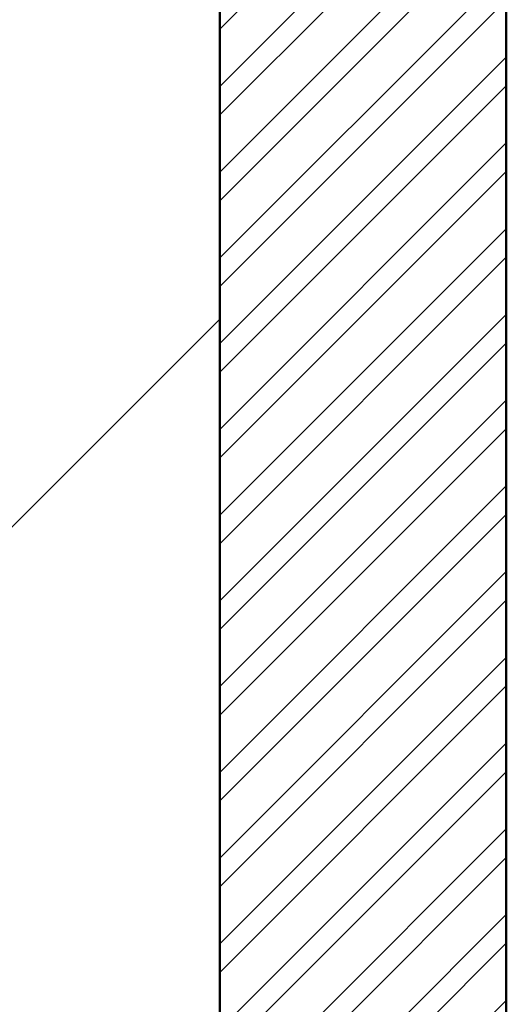
# Model space of a CAD drawing. Units: inches. Extents: x 3590 to 5167, y 65 to 1917.
# Tile 43 of 100: x 5065 to 5080, y 1357 to 1388. Entities that reach past the tile are written whole.
import ezdxf

# ---------------------------------------------------------------- set-up
doc = ezdxf.new("R2010")
doc.units = ezdxf.units.IN
for name, color, linetype, lineweight in [('A-FLOR-PATT', 8, 'Continuous', 13), ('A-WALL', 7, 'Continuous', 50), ('A-WALL-PATT', 251, 'Continuous', 13)]:
    doc.layers.add(name, color=color, linetype=linetype, lineweight=lineweight)

msp = doc.modelspace()

# ---------------------------------------------------------------- hatches: boundary and pattern name
at = {"layer": 'A-FLOR-PATT', "transparency": 33554687}
h = msp.add_hatch(dxfattribs=at)
h.set_pattern_fill('AR-HBONE', color=256, scale=0.2)
h.set_pattern_definition([(45, (-588.972, 0), (0, 28.73682), [60.96, -20.32]), (135, (-574.604, 14.368), (3e-15, 28.73682), [60.96, -20.32])])
h.paths.add_polyline_path([(5071.274, 1796.999), (4933.274, 1796.999), (4933.274, 1753.999), (4962.774, 1753.999, -0.414214), (4928.774, 1719.999), (4933.274, 1718.999), (4933.274, 1334.999), (5071.274, 1334.999)])
h.paths.add_polyline_path([(4951.78, 1521.077), (4951.715, 1521.04), (4951.563, 1520.895)], flags=16)
h.paths.add_polyline_path([(4952.267, 1521.376), (4952.198, 1521.371), (4952.198, 1521.356)], flags=0)
h.paths.add_polyline_path([(4967.051, 1529.728), (4965.231, 1528.694), (4963.411, 1527.714), (4961.756, 1526.851), (4963.589, 1527.449), (4964.036, 1527.478), (4962.975, 1527.249), (4961.76, 1526.852), (4959.792, 1525.834), (4958.005, 1524.895), (4956.24, 1523.93), (4954.504, 1522.919), (4954.129, 1522.682), (4953.361, 1521.997), (4953.366, 1521.998), (4953.605, 1522.064), (4955.106, 1522.761), (4956.921, 1523.434), (4958.678, 1523.915), (4960.358, 1524.2), (4961.945, 1524.286), (4964.171, 1524.108), (4965.958, 1523.309), (4963.863, 1522.976), (4965.187, 1522.499), (4963.366, 1522.497), (4961.545, 1522.487), (4959.764, 1522.461), (4958.304, 1522.419), (4957.974, 1522.388), (4956.307, 1522.232), (4954.718, 1522.071), (4953.251, 1521.899), (4953.525, 1521.623), (4954.331, 1521.379), (4956.243, 1521.23), (4958.039, 1520.93), (4959.684, 1520.483), (4961.16, 1519.896), (4963.107, 1518.8), (4964.393, 1517.325), (4962.973, 1517.726), (4964.558, 1516.661), (4965.407, 1515.708), (4963.507, 1516.322), (4961.68, 1517.005), (4959.935, 1517.745), (4958.282, 1518.528), (4956.732, 1519.343), (4955.295, 1520.175), (4954.672, 1520.572), (4954.513, 1520.627), (4955.658, 1519.318), (4956.703, 1517.982), (4957.644, 1516.647), (4958.485, 1515.334), (4959.55, 1513.524), (4960.438, 1511.769), (4958.841, 1513.62), (4957.452, 1515.325), (4955.819, 1517.459), (4956.665, 1515.448), (4957.111, 1513.923), (4957.447, 1511.714), (4957.076, 1509.793), (4956.538, 1511.11), (4955.992, 1512.569), (4955.444, 1514.125), (4954.898, 1515.735), (4954.357, 1517.356), (4953.824, 1518.943), (4953.305, 1520.452), (4953.065, 1521.116), (4952.971, 1521.146), (4952.949, 1521.086), (4952.73, 1520.199), (4953.37, 1518.024), (4953.757, 1516.373), (4954.051, 1514.765), (4954.264, 1513.221), (4954.471, 1511.131), (4954.497, 1510.402), (4954.409, 1511.76), (4954.264, 1513.221), (4954.051, 1514.765), (4953.757, 1516.373), (4953.37, 1518.024), (4952.877, 1519.698), (4952.716, 1520.141), (4952.533, 1519.059), (4952.374, 1517.789), (4952.219, 1516.312), (4952.046, 1514.6), (4951.833, 1512.626), (4951.557, 1510.363), (4951.203, 1512.168), (4950.852, 1514.339), (4950.985, 1516.376), (4951.66, 1518.286), (4952.593, 1520.481), (4952.357, 1521.13), (4951.855, 1520.328), (4950.839, 1518.908), (4949.777, 1517.587), (4948.916, 1516.617), (4948.111, 1515.256), (4947.089, 1513.554), (4945.889, 1511.615), (4946.326, 1513.402), (4946.562, 1514.249), (4945.528, 1513.327), (4944.581, 1512.531), (4946.018, 1514.508), (4947.204, 1516.048), (4947.893, 1517.313), (4949.307, 1518.764), (4950.414, 1519.767), (4950.451, 1519.806), (4952.267, 1521.376), (4951.645, 1521.493), (4950.404, 1521.18), (4948.044, 1520.359), (4946.119, 1519.452), (4944.572, 1518.475), (4943.35, 1517.443), (4941.997, 1515.92), (4941.661, 1515.275), (4942.813, 1516.99), (4944.572, 1518.475), (4946.119, 1519.452), (4948.044, 1520.359), (4950.404, 1521.18), (4951.645, 1521.493), (4949.647, 1521.868), (4948.6, 1521.756), (4947.126, 1521.57), (4945.42, 1521.348), (4943.45, 1521.105), (4941.183, 1520.856), (4942.86, 1521.613), (4943.873, 1522.03), (4942.952, 1521.909), (4941.41, 1521.485), (4939.543, 1520.67), (4938.968, 1520.226), (4940.733, 1521.299), (4942.952, 1521.909), (4943.702, 1522.008), (4945.894, 1522.7), (4947.565, 1522.714), (4948.921, 1522.566), (4951.131, 1522.183), (4950.971, 1522.297), (4948.129, 1523.006), (4946.035, 1523.707), (4944.232, 1524.521), (4942.707, 1525.461), (4941.444, 1526.537), (4940.43, 1527.761), (4939.649, 1529.143), (4941.421, 1528.122), (4943.147, 1527.132), (4944.841, 1526.175), (4946.514, 1525.25), (4948.179, 1524.359), (4948.365, 1524.263), (4946.475, 1526.045), (4945.181, 1527.54), (4944.19, 1529.033), (4943.496, 1530.54), (4943.278, 1531.36), (4942.498, 1531.919), (4943.114, 1531.762), (4942.959, 1533.659), (4944.14, 1531.989), (4944.612, 1531.323), (4946.202, 1530.463), (4947.486, 1529.509), (4948.79, 1528.226), (4950.368, 1526.237), (4949.485, 1528.155), (4948.851, 1530.123), (4948.491, 1532.041), (4948.381, 1533.918), (4948.501, 1535.76), (4948.827, 1537.573), (4949.418, 1535.565), (4949.957, 1533.569), (4950.464, 1531.586), (4950.961, 1529.617), (4951.391, 1527.954), (4951.724, 1530.687), (4952.201, 1532.58), (4952.889, 1534.33), (4953.77, 1535.951), (4954.827, 1537.46), (4954.521, 1535.39), (4954.273, 1533.937), (4955.58, 1535.663), (4956.748, 1536.739), (4956.159, 1534.78), (4955.589, 1532.873), (4955.043, 1531.006), (4954.525, 1529.166), (4954.038, 1527.341), (4953.638, 1525.733), (4953.611, 1525.586), (4953.398, 1524.166), (4953.382, 1524.009), (4954.07, 1525.476), (4954.912, 1527.022), (4956.136, 1528.894), (4957.847, 1530.577), (4959.376, 1531.54), (4958.256, 1530.104), (4957.143, 1528.663), (4956.066, 1527.243), (4955.056, 1525.871), (4954.141, 1524.571), (4953.352, 1523.372), (4953.311, 1523.303), (4953.273, 1522.925), (4953.261, 1522.382), (4954.103, 1523.373), (4954.63, 1524.284), (4955.961, 1526.358), (4957.23, 1528.13), (4958.421, 1529.609), (4960.037, 1531.368), (4961.374, 1532.375), (4962.101, 1532.77), (4961.07, 1531.061), (4959.987, 1529.438), (4958.869, 1527.908), (4958.15, 1527.007), (4959.803, 1528.003), (4961.589, 1528.793), (4963.391, 1529.328), (4965.211, 1529.632)], flags=16)
h.paths.add_polyline_path([(4962.944, 1523.182), (4961.107, 1523.422), (4960.392, 1523.362), (4962.35, 1523.331)], flags=0)
h.paths.add_polyline_path([(5049.541, 1584.551), (5049.476, 1584.515), (5049.325, 1584.37)], flags=16)
h.paths.add_polyline_path([(5050.028, 1584.851), (5049.959, 1584.845), (5049.959, 1584.83)], flags=0)
h.paths.add_polyline_path([(5042.333, 1581.949), (5043.88, 1582.926), (5045.806, 1583.833), (5048.165, 1584.654), (5049.406, 1584.967), (5047.408, 1585.342), (5046.361, 1585.231), (5044.888, 1585.044), (5043.181, 1584.822), (5041.211, 1584.579), (5038.944, 1584.33), (5040.622, 1585.087), (5041.634, 1585.504), (5040.713, 1585.383), (5039.171, 1584.959), (5037.304, 1584.144), (5036.729, 1583.7), (5038.494, 1584.773), (5040.713, 1585.383), (5041.463, 1585.482), (5043.655, 1586.174), (5045.326, 1586.188), (5046.682, 1586.04), (5048.893, 1585.657), (5048.732, 1585.771), (5045.891, 1586.48), (5043.796, 1587.181), (5041.994, 1587.996), (5040.468, 1588.935), (5039.205, 1590.011), (5038.191, 1591.235), (5037.41, 1592.617), (5039.182, 1591.596), (5040.909, 1590.607), (5042.602, 1589.649), (5044.275, 1588.724), (5045.94, 1587.833), (5046.126, 1587.738), (5044.237, 1589.519), (5042.942, 1591.015), (5041.952, 1592.508), (5041.257, 1594.014), (5041.039, 1594.834), (5040.26, 1595.393), (5040.875, 1595.237), (5040.721, 1597.133), (5041.901, 1595.463), (5042.373, 1594.798), (5043.963, 1593.938), (5045.247, 1592.983), (5046.552, 1591.701), (5048.129, 1589.712), (5047.247, 1591.63), (5046.613, 1593.597), (5046.252, 1595.515), (5046.142, 1597.392), (5046.262, 1599.234), (5046.588, 1601.047), (5047.179, 1599.039), (5047.718, 1597.043), (5048.225, 1595.06), (5048.722, 1593.091), (5049.152, 1591.429), (5049.485, 1594.161), (5049.962, 1596.054), (5050.65, 1597.804), (5051.532, 1599.425), (5052.589, 1600.934), (5052.283, 1598.864), (5052.034, 1597.411), (5053.341, 1599.137), (5054.509, 1600.213), (5053.92, 1598.254), (5053.35, 1596.348), (5052.805, 1594.48), (5052.286, 1592.64), (5051.799, 1590.815), (5051.4, 1589.207), (5051.373, 1589.06), (5051.159, 1587.64), (5051.143, 1587.483), (5051.831, 1588.95), (5052.673, 1590.496), (5053.898, 1592.368), (5055.608, 1594.051), (5057.137, 1595.014), (5056.017, 1593.578), (5054.904, 1592.137), (5053.828, 1590.717), (5052.817, 1589.345), (5051.902, 1588.046), (5051.113, 1586.846), (5051.072, 1586.777), (5051.034, 1586.399), (5051.022, 1585.856), (5051.864, 1586.847), (5052.391, 1587.758), (5053.723, 1589.832), (5054.991, 1591.604), (5056.182, 1593.083), (5057.798, 1594.842), (5059.135, 1595.849), (5059.863, 1596.244), (5058.831, 1594.535), (5057.749, 1592.912), (5056.63, 1591.382), (5055.912, 1590.482), (5057.564, 1591.477), (5059.35, 1592.267), (5061.152, 1592.802), (5062.972, 1593.106), (5064.812, 1593.203), (5062.992, 1592.169), (5061.172, 1591.188), (5059.518, 1590.325), (5061.35, 1590.924), (5061.797, 1590.952), (5060.737, 1590.723), (5059.521, 1590.326), (5057.553, 1589.308), (5055.766, 1588.369), (5054.002, 1587.404), (5052.265, 1586.393), (5051.891, 1586.156), (5051.122, 1585.471), (5051.127, 1585.472), (5051.366, 1585.538), (5052.867, 1586.235), (5054.682, 1586.908), (5056.439, 1587.389), (5058.12, 1587.675), (5059.706, 1587.76), (5061.933, 1587.583), (5063.719, 1586.783), (5061.624, 1586.45), (5062.949, 1585.973), (5061.127, 1585.971), (5059.307, 1585.961), (5057.525, 1585.935), (5056.065, 1585.893), (5055.735, 1585.862), (5054.068, 1585.707), (5052.479, 1585.546), (5051.012, 1585.373), (5051.286, 1585.097), (5052.092, 1584.853), (5054.004, 1584.704), (5055.8, 1584.404), (5057.446, 1583.958), (5058.921, 1583.37), (5060.868, 1582.274), (5062.154, 1580.799), (5060.734, 1581.2), (5062.32, 1580.135), (5063.168, 1579.182), (5061.269, 1579.796), (5059.441, 1580.479), (5057.696, 1581.219), (5056.043, 1582.003), (5054.493, 1582.817), (5053.057, 1583.649), (5052.433, 1584.047), (5052.274, 1584.101), (5053.42, 1582.793), (5054.464, 1581.457), (5055.405, 1580.121), (5056.247, 1578.809), (5057.311, 1576.998), (5058.199, 1575.244), (5056.602, 1577.094), (5055.213, 1578.799), (5053.58, 1580.933), (5054.427, 1578.922), (5054.872, 1577.397), (5055.208, 1575.189), (5054.838, 1573.267), (5054.299, 1574.584), (5053.754, 1576.043), (5053.206, 1577.599), (5052.659, 1579.209), (5052.118, 1580.83), (5051.585, 1582.417), (5051.066, 1583.927), (5050.826, 1584.59), (5050.733, 1584.62), (5050.711, 1584.561), (5050.491, 1583.673), (5051.131, 1581.498), (5051.518, 1579.847), (5051.813, 1578.24), (5052.026, 1576.695), (5052.233, 1574.605), (5052.258, 1573.876), (5052.17, 1575.234), (5052.026, 1576.695), (5051.813, 1578.24), (5051.518, 1579.847), (5051.131, 1581.498), (5050.638, 1583.172), (5050.477, 1583.615), (5050.294, 1582.533), (5050.136, 1581.263), (5049.981, 1579.786), (5049.807, 1578.074), (5049.594, 1576.1), (5049.318, 1573.837), (5048.965, 1575.642), (5048.613, 1577.813), (5048.747, 1579.85), (5049.421, 1581.76), (5050.354, 1583.955), (5050.118, 1584.604), (5049.616, 1583.802), (5048.6, 1582.382), (5047.538, 1581.061), (5046.677, 1580.091), (5045.872, 1578.73), (5044.85, 1577.028), (5043.651, 1575.089), (5044.087, 1576.877), (5044.324, 1577.723), (5043.289, 1576.801), (5042.342, 1576.005), (5043.779, 1577.982), (5044.966, 1579.522), (5045.655, 1580.787), (5047.068, 1582.239), (5048.175, 1583.241), (5048.213, 1583.28), (5050.028, 1584.851), (5049.406, 1584.967), (5048.165, 1584.654), (5045.806, 1583.833), (5043.88, 1582.926), (5042.333, 1581.949), (5041.111, 1580.917), (5039.758, 1579.394), (5039.423, 1578.749), (5040.575, 1580.464)], flags=16)
h.paths.add_polyline_path([(4954.799, 1533.12), (4954.262, 1532.079), (4953.831, 1530.935), (4953.505, 1529.636), (4953.283, 1528.133), (4953.167, 1526.376), (4953.156, 1524.315), (4953.277, 1521.236), (4952.802, 1521.842), (4951.557, 1521.998), (4950.976, 1521.961), (4952.661, 1521.941), (4952.802, 1521.842), (4953.152, 1523.593), (4953.167, 1526.376), (4953.283, 1528.133), (4953.609, 1530.346), (4954.456, 1532.592)], flags=0)
h.paths.add_polyline_path([(5050.563, 1585.316), (5049.318, 1585.472), (5048.737, 1585.435), (5050.422, 1585.415), (5050.563, 1585.316), (5050.914, 1587.067), (5050.928, 1589.851), (5051.045, 1591.607), (5051.371, 1593.82), (5052.217, 1596.066), (5052.56, 1596.594), (5052.024, 1595.554), (5051.592, 1594.409), (5051.266, 1593.11), (5051.045, 1591.607), (5050.928, 1589.851), (5050.918, 1587.789), (5051.038, 1584.71)], flags=0)
h.paths.add_polyline_path([(5058.153, 1586.836), (5060.111, 1586.805), (5060.705, 1586.656), (5058.868, 1586.896)], flags=0)
h.paths.add_polyline_path([(5049.541, 1430.936), (5049.476, 1430.9), (5049.325, 1430.755)], flags=16)
h.paths.add_polyline_path([(5050.028, 1431.236), (5049.959, 1431.231), (5049.959, 1431.215)], flags=0)
h.paths.add_polyline_path([(5046.588, 1447.432), (5047.179, 1445.425), (5047.718, 1443.429), (5048.225, 1441.446), (5048.722, 1439.476), (5049.152, 1437.814), (5049.485, 1440.546), (5049.962, 1442.439), (5050.65, 1444.189), (5051.532, 1445.811), (5052.589, 1447.319), (5052.283, 1445.249), (5052.034, 1443.796), (5053.341, 1445.522), (5054.509, 1446.598), (5053.92, 1444.64), (5053.35, 1442.733), (5052.805, 1440.865), (5052.286, 1439.025), (5051.799, 1437.201), (5051.4, 1435.592), (5051.373, 1435.445), (5051.159, 1434.025), (5051.143, 1433.868), (5051.831, 1435.335), (5052.673, 1436.881), (5053.898, 1438.753), (5055.608, 1440.436), (5057.137, 1441.4), (5056.017, 1439.963), (5054.904, 1438.522), (5053.828, 1437.102), (5052.817, 1435.73), (5051.902, 1434.431), (5051.113, 1433.231), (5051.072, 1433.162), (5051.034, 1432.784), (5051.022, 1432.242), (5051.864, 1433.232), (5052.391, 1434.143), (5053.723, 1436.217), (5054.991, 1437.989), (5056.182, 1439.468), (5057.798, 1441.227), (5059.135, 1442.235), (5059.863, 1442.629), (5058.831, 1440.921), (5057.749, 1439.298), (5056.63, 1437.767), (5055.912, 1436.867), (5057.564, 1437.863), (5059.35, 1438.652), (5061.152, 1439.187), (5062.972, 1439.491), (5064.812, 1439.588), (5062.992, 1438.554), (5061.172, 1437.573), (5059.518, 1436.71), (5061.35, 1437.309), (5061.797, 1437.337), (5060.737, 1437.108), (5059.521, 1436.711), (5057.553, 1435.693), (5055.766, 1434.754), (5054.002, 1433.789), (5052.265, 1432.778), (5051.891, 1432.541), (5051.122, 1431.856), (5051.127, 1431.857), (5051.366, 1431.923), (5052.867, 1432.62), (5054.682, 1433.293), (5056.439, 1433.775), (5058.12, 1434.06), (5059.706, 1434.145), (5061.933, 1433.968), (5063.719, 1433.168), (5061.624, 1432.835), (5062.949, 1432.358), (5061.127, 1432.357), (5059.307, 1432.346), (5057.525, 1432.32), (5056.065, 1432.278), (5055.735, 1432.248), (5054.068, 1432.092), (5052.479, 1431.931), (5051.012, 1431.759), (5051.286, 1431.482), (5052.092, 1431.238), (5054.004, 1431.089), (5055.8, 1430.789), (5057.446, 1430.343), (5058.921, 1429.755), (5060.868, 1428.66), (5062.154, 1427.185), (5060.734, 1427.585), (5062.32, 1426.52), (5063.168, 1425.567), (5061.269, 1426.181), (5059.441, 1426.865), (5057.696, 1427.604), (5056.043, 1428.388), (5054.493, 1429.202), (5053.057, 1430.034), (5052.433, 1430.432), (5052.274, 1430.487), (5053.42, 1429.178), (5054.464, 1427.842), (5055.405, 1426.506), (5056.247, 1425.194), (5057.311, 1423.383), (5058.199, 1421.629), (5056.602, 1423.479), (5055.213, 1425.184), (5053.58, 1427.318), (5054.427, 1425.307), (5054.872, 1423.782), (5055.208, 1421.574), (5054.838, 1419.652), (5054.299, 1420.97), (5053.754, 1422.428), (5053.206, 1423.984), (5052.659, 1425.595), (5052.118, 1427.215), (5051.585, 1428.802), (5051.066, 1430.312), (5050.826, 1430.975), (5050.733, 1431.005), (5050.711, 1430.946), (5050.491, 1430.058), (5051.131, 1427.883), (5051.518, 1426.232), (5051.813, 1424.625), (5052.026, 1423.081), (5052.233, 1420.991), (5052.258, 1420.261), (5052.17, 1421.619), (5052.026, 1423.081), (5051.813, 1424.625), (5051.518, 1426.232), (5051.131, 1427.883), (5050.638, 1429.558), (5050.477, 1430.001), (5050.294, 1428.918), (5050.136, 1427.648), (5049.981, 1426.171), (5049.807, 1424.459), (5049.594, 1422.485), (5049.318, 1420.222), (5048.965, 1422.028), (5048.613, 1424.199), (5048.747, 1426.235), (5049.421, 1428.146), (5050.354, 1430.34), (5050.118, 1430.989), (5049.616, 1430.187), (5048.6, 1428.768), (5047.538, 1427.446), (5046.677, 1426.477), (5045.872, 1425.116), (5044.85, 1423.413), (5043.651, 1421.474), (5044.087, 1423.262), (5044.324, 1424.109), (5043.289, 1423.186), (5042.342, 1422.391), (5043.779, 1424.368), (5044.966, 1425.907), (5045.655, 1427.173), (5047.068, 1428.624), (5048.175, 1429.627), (5048.213, 1429.666), (5050.028, 1431.236), (5049.406, 1431.353), (5048.165, 1431.039), (5045.806, 1430.218), (5043.88, 1429.311), (5042.333, 1428.334), (5041.111, 1427.302), (5039.758, 1425.779), (5039.423, 1425.134), (5040.575, 1426.849), (5042.333, 1428.334), (5043.88, 1429.311), (5045.806, 1430.218), (5048.165, 1431.039), (5049.406, 1431.353), (5047.408, 1431.727), (5046.361, 1431.616), (5044.888, 1431.429), (5043.181, 1431.207), (5041.211, 1430.964), (5038.944, 1430.715), (5040.622, 1431.472), (5041.634, 1431.89), (5040.713, 1431.769), (5039.171, 1431.345), (5037.304, 1430.53), (5036.729, 1430.085), (5038.494, 1431.158), (5040.713, 1431.769), (5041.463, 1431.867), (5043.655, 1432.559), (5045.326, 1432.573), (5046.682, 1432.425), (5048.893, 1432.042), (5048.732, 1432.156), (5045.891, 1432.865), (5043.796, 1433.566), (5041.994, 1434.381), (5040.468, 1435.321), (5039.205, 1436.396), (5038.191, 1437.62), (5037.41, 1439.002), (5039.182, 1437.982), (5040.909, 1436.992), (5042.602, 1436.034), (5044.275, 1435.109), (5045.94, 1434.218), (5046.126, 1434.123), (5044.237, 1435.904), (5042.942, 1437.4), (5041.952, 1438.893), (5041.257, 1440.399), (5041.039, 1441.219), (5040.26, 1441.778), (5040.875, 1441.622), (5040.721, 1443.518), (5041.901, 1441.848), (5042.373, 1441.183), (5043.963, 1440.323), (5045.247, 1439.369), (5046.552, 1438.086), (5048.129, 1436.097), (5047.247, 1438.015), (5046.613, 1439.982), (5046.252, 1441.901), (5046.142, 1443.778), (5046.262, 1445.619)], flags=16)
h.paths.add_polyline_path([(5052.382, 1444.255), (5051.623, 1442.78), (5052.024, 1441.939), (5052.56, 1442.98)], flags=0)
h.paths.add_polyline_path([(5050.563, 1431.701), (5049.318, 1431.857), (5048.737, 1431.821), (5050.422, 1431.8)], flags=0)
h.paths.add_polyline_path([(5058.153, 1433.221), (5060.111, 1433.19), (5060.705, 1433.041), (5058.868, 1433.281)], flags=0)
h.paths.add_polyline_path([(5049.541, 1352.285), (5049.476, 1352.249), (5049.325, 1352.104)], flags=16)
h.paths.add_polyline_path([(5050.028, 1352.585), (5049.959, 1352.58), (5049.959, 1352.564)], flags=0)
h.paths.add_polyline_path([(5046.588, 1368.781), (5047.179, 1366.774), (5047.718, 1364.778), (5048.225, 1362.795), (5048.722, 1360.825), (5049.152, 1359.163), (5049.485, 1361.896), (5049.962, 1363.789), (5050.65, 1365.538), (5051.532, 1367.16), (5052.589, 1368.669), (5052.283, 1366.598), (5052.034, 1365.145), (5053.341, 1366.871), (5054.509, 1367.947), (5053.92, 1365.989), (5053.35, 1364.082), (5052.805, 1362.214), (5052.286, 1360.374), (5051.799, 1358.55), (5051.4, 1356.942), (5051.373, 1356.794), (5051.159, 1355.374), (5051.143, 1355.218), (5051.831, 1356.684), (5052.673, 1358.23), (5053.898, 1360.102), (5055.608, 1361.786), (5057.137, 1362.749), (5056.017, 1361.313), (5054.904, 1359.872), (5053.828, 1358.452), (5052.817, 1357.079), (5051.902, 1355.78), (5051.113, 1354.581), (5051.072, 1354.512), (5051.034, 1354.133), (5051.022, 1353.591), (5051.864, 1354.581), (5052.391, 1355.492), (5053.723, 1357.566), (5054.991, 1359.338), (5056.182, 1360.817), (5057.798, 1362.577), (5059.135, 1363.584), (5059.863, 1363.979), (5058.831, 1362.27), (5057.749, 1360.647), (5056.63, 1359.117), (5055.912, 1358.216), (5057.564, 1359.212), (5059.35, 1360.001), (5061.152, 1360.536), (5062.972, 1360.841), (5064.812, 1360.937), (5062.992, 1359.903), (5061.172, 1358.923), (5059.518, 1358.059), (5061.35, 1358.658), (5061.797, 1358.687), (5060.737, 1358.458), (5059.521, 1358.061), (5057.553, 1357.043), (5055.766, 1356.103), (5054.002, 1355.138), (5052.265, 1354.127), (5051.891, 1353.89), (5051.122, 1353.206), (5051.127, 1353.206), (5051.366, 1353.272), (5052.867, 1353.969), (5054.682, 1354.643), (5056.439, 1355.124), (5058.12, 1355.409), (5059.706, 1355.495), (5061.933, 1355.317), (5063.719, 1354.518), (5061.624, 1354.184), (5062.949, 1353.708), (5061.127, 1353.706), (5059.307, 1353.695), (5057.525, 1353.669), (5056.065, 1353.627), (5055.735, 1353.597), (5054.068, 1353.441), (5052.479, 1353.28), (5051.012, 1353.108), (5051.286, 1352.831), (5052.092, 1352.587), (5054.004, 1352.439), (5055.8, 1352.138), (5057.446, 1351.692), (5058.921, 1351.104), (5060.868, 1350.009), (5062.154, 1348.534), (5060.734, 1348.935), (5062.32, 1347.869), (5063.168, 1346.916), (5061.269, 1347.53), (5059.441, 1348.214), (5057.696, 1348.954), (5056.043, 1349.737), (5054.493, 1350.551), (5053.057, 1351.383), (5052.433, 1351.781), (5052.274, 1351.836), (5053.42, 1350.527), (5054.464, 1349.191), (5055.405, 1347.855), (5056.247, 1346.543), (5057.311, 1344.733), (5058.199, 1342.978), (5056.602, 1344.828), (5055.213, 1346.534), (5053.58, 1348.667), (5054.427, 1346.656), (5054.872, 1345.132), (5055.208, 1342.923), (5054.838, 1341.002), (5054.299, 1342.319), (5053.754, 1343.778), (5053.206, 1345.334), (5052.659, 1346.944), (5052.118, 1348.564), (5051.585, 1350.151), (5051.066, 1351.661), (5050.826, 1352.324), (5050.733, 1352.355), (5050.711, 1352.295), (5050.491, 1351.408), (5051.131, 1349.232), (5051.518, 1347.581), (5051.813, 1345.974), (5052.026, 1344.43), (5052.233, 1342.34), (5052.258, 1341.61), (5052.17, 1342.969), (5052.026, 1344.43), (5051.813, 1345.974), (5051.518, 1347.581), (5051.131, 1349.232), (5050.638, 1350.907), (5050.477, 1351.35), (5050.294, 1350.267), (5050.136, 1348.997), (5049.981, 1347.52), (5049.807, 1345.809), (5049.594, 1343.835), (5049.318, 1341.571), (5048.965, 1343.377), (5048.613, 1345.548), (5048.747, 1347.585), (5049.421, 1349.495), (5050.354, 1351.689), (5050.118, 1352.339), (5049.616, 1351.536), (5048.6, 1350.117), (5047.538, 1348.795), (5046.677, 1347.826), (5045.872, 1346.465), (5044.85, 1344.763), (5043.651, 1342.824), (5044.087, 1344.611), (5044.324, 1345.458), (5043.289, 1344.535), (5042.342, 1343.74), (5043.779, 1345.717), (5044.966, 1347.256), (5045.655, 1348.522), (5047.068, 1349.973), (5048.175, 1350.976), (5048.213, 1351.015), (5050.028, 1352.585), (5049.406, 1352.702), (5048.165, 1352.388), (5045.806, 1351.567), (5043.88, 1350.661), (5042.333, 1349.683), (5041.111, 1348.651), (5039.758, 1347.128), (5039.423, 1346.483), (5040.575, 1348.198), (5042.333, 1349.683), (5043.88, 1350.661), (5045.806, 1351.567), (5048.165, 1352.388), (5049.406, 1352.702), (5047.408, 1353.076), (5046.361, 1352.965), (5044.888, 1352.779), (5043.181, 1352.556), (5041.211, 1352.313), (5038.944, 1352.065), (5040.622, 1352.821), (5041.634, 1353.239), (5040.713, 1353.118), (5039.171, 1352.694), (5037.304, 1351.879), (5036.729, 1351.434), (5038.494, 1352.508), (5040.713, 1353.118), (5041.463, 1353.216), (5043.655, 1353.909), (5045.326, 1353.923), (5046.682, 1353.774), (5048.893, 1353.391), (5048.732, 1353.506), (5045.891, 1354.214), (5043.796, 1354.915), (5041.994, 1355.73), (5040.468, 1356.67), (5039.205, 1357.746), (5038.191, 1358.969), (5037.41, 1360.352), (5039.182, 1359.331), (5040.909, 1358.341), (5042.602, 1357.383), (5044.275, 1356.458), (5045.94, 1355.567), (5046.126, 1355.472), (5044.237, 1357.253), (5042.942, 1358.749), (5041.952, 1360.242), (5041.257, 1361.748), (5041.039, 1362.568), (5040.26, 1363.128), (5040.875, 1362.971), (5040.721, 1364.867), (5041.901, 1363.197), (5042.373, 1362.532), (5043.963, 1361.672), (5045.247, 1360.718), (5046.552, 1359.435), (5048.129, 1357.446), (5047.247, 1359.364), (5046.613, 1361.331), (5046.252, 1363.25), (5046.142, 1365.127), (5046.262, 1366.969)], flags=16)
h.paths.add_polyline_path([(5052.382, 1365.604), (5051.623, 1364.129), (5052.024, 1363.288), (5052.56, 1364.329)], flags=0)
h.paths.add_polyline_path([(4951.78, 1698.041), (4951.715, 1698.005), (4951.563, 1697.859)], flags=16)
h.paths.add_polyline_path([(4952.267, 1698.341), (4952.198, 1698.335), (4952.198, 1698.32)], flags=0)
h.paths.add_polyline_path([(4957.076, 1686.757), (4956.538, 1688.074), (4955.992, 1689.533), (4955.444, 1691.089), (4954.898, 1692.699), (4954.357, 1694.32), (4953.824, 1695.907), (4953.305, 1697.417), (4953.065, 1698.08), (4952.971, 1698.11), (4952.949, 1698.051), (4952.73, 1697.163), (4953.37, 1694.988), (4953.757, 1693.337), (4954.051, 1691.729), (4954.264, 1690.185), (4954.471, 1688.095), (4954.497, 1687.366), (4954.409, 1688.724), (4954.264, 1690.185), (4954.051, 1691.729), (4953.757, 1693.337), (4953.37, 1694.988), (4952.877, 1696.662), (4952.716, 1697.105), (4952.533, 1696.023), (4952.374, 1694.753), (4952.219, 1693.276), (4952.046, 1691.564), (4951.833, 1689.59), (4951.557, 1687.327), (4951.203, 1689.132), (4950.852, 1691.303), (4950.985, 1693.34), (4951.66, 1695.25), (4952.593, 1697.445), (4952.357, 1698.094), (4951.855, 1697.292), (4950.839, 1695.872), (4949.777, 1694.551), (4948.916, 1693.581), (4948.111, 1692.22), (4947.089, 1690.518), (4945.889, 1688.579), (4946.326, 1690.366), (4946.562, 1691.213), (4945.528, 1690.291), (4944.581, 1689.495), (4946.018, 1691.472), (4947.204, 1693.012), (4947.893, 1694.277), (4949.307, 1695.729), (4950.414, 1696.731), (4950.451, 1696.77), (4952.267, 1698.341), (4951.645, 1698.457), (4950.404, 1698.144), (4948.044, 1697.323), (4946.119, 1696.416), (4944.572, 1695.439), (4943.35, 1694.407), (4941.997, 1692.884), (4941.661, 1692.239), (4942.813, 1693.954), (4944.572, 1695.439), (4946.119, 1696.416), (4948.044, 1697.323), (4950.404, 1698.144), (4951.645, 1698.457), (4949.647, 1698.832), (4948.6, 1698.72), (4947.126, 1698.534), (4945.42, 1698.312), (4943.45, 1698.069), (4941.183, 1697.82), (4942.86, 1698.577), (4943.873, 1698.994), (4942.952, 1698.873), (4941.41, 1698.449), (4939.543, 1697.634), (4938.968, 1697.19), (4940.733, 1698.263), (4942.952, 1698.873), (4943.702, 1698.972), (4945.894, 1699.664), (4947.565, 1699.678), (4948.921, 1699.53), (4951.131, 1699.147), (4950.971, 1699.261), (4948.129, 1699.97), (4946.035, 1700.671), (4944.232, 1701.486), (4942.707, 1702.425), (4941.444, 1703.501), (4940.43, 1704.725), (4939.649, 1706.107), (4941.421, 1705.086), (4943.147, 1704.097), (4944.841, 1703.139), (4946.514, 1702.214), (4948.179, 1701.323), (4948.365, 1701.227), (4946.475, 1703.009), (4945.181, 1704.505), (4944.19, 1705.997), (4943.496, 1707.504), (4943.278, 1708.324), (4942.498, 1708.883), (4943.114, 1708.727), (4942.959, 1710.623), (4944.14, 1708.953), (4944.612, 1708.287), (4946.202, 1707.428), (4947.486, 1706.473), (4948.79, 1705.191), (4950.368, 1703.202), (4949.485, 1705.12), (4948.851, 1707.087), (4948.491, 1709.005), (4948.381, 1710.882), (4948.501, 1712.724), (4948.827, 1714.537), (4949.418, 1712.529), (4949.957, 1710.533), (4950.464, 1708.55), (4950.961, 1706.581), (4951.391, 1704.919), (4951.724, 1707.651), (4952.201, 1709.544), (4952.889, 1711.294), (4953.77, 1712.915), (4954.827, 1714.424), (4954.521, 1712.354), (4954.273, 1710.901), (4955.58, 1712.627), (4956.748, 1713.703), (4956.159, 1711.744), (4955.589, 1709.837), (4955.043, 1707.97), (4954.525, 1706.13), (4954.038, 1704.305), (4953.638, 1702.697), (4953.611, 1702.55), (4953.398, 1701.13), (4953.382, 1700.973), (4954.07, 1702.44), (4954.912, 1703.986), (4956.136, 1705.858), (4957.847, 1707.541), (4959.376, 1708.504), (4958.256, 1707.068), (4957.143, 1705.627), (4956.066, 1704.207), (4955.056, 1702.835), (4954.141, 1701.536), (4953.352, 1700.336), (4953.311, 1700.267), (4953.273, 1699.889), (4953.261, 1699.346), (4954.103, 1700.337), (4954.63, 1701.248), (4955.961, 1703.322), (4957.23, 1705.094), (4958.421, 1706.573), (4960.037, 1708.332), (4961.374, 1709.339), (4962.101, 1709.734), (4961.07, 1708.025), (4959.987, 1706.402), (4958.869, 1704.872), (4958.15, 1703.972), (4959.803, 1704.967), (4961.589, 1705.757), (4963.391, 1706.292), (4965.211, 1706.596), (4967.051, 1706.692), (4965.231, 1705.659), (4963.411, 1704.678), (4961.756, 1703.815), (4963.589, 1704.413), (4964.036, 1704.442), (4962.975, 1704.213), (4961.76, 1703.816), (4959.792, 1702.798), (4958.005, 1701.859), (4956.24, 1700.894), (4954.504, 1699.883), (4954.129, 1699.646), (4953.361, 1698.961), (4953.366, 1698.962), (4953.605, 1699.028), (4955.106, 1699.725), (4956.921, 1700.398), (4958.678, 1700.879), (4960.358, 1701.164), (4961.945, 1701.25), (4964.171, 1701.073), (4965.958, 1700.273), (4963.863, 1699.94), (4965.187, 1699.463), (4963.366, 1699.461), (4961.545, 1699.451), (4959.764, 1699.425), (4958.304, 1699.383), (4957.974, 1699.352), (4956.307, 1699.197), (4954.718, 1699.036), (4953.251, 1698.863), (4953.525, 1698.587), (4954.331, 1698.343), (4956.243, 1698.194), (4958.039, 1697.894), (4959.684, 1697.447), (4961.16, 1696.86), (4963.107, 1695.764), (4964.393, 1694.289), (4962.973, 1694.69), (4964.558, 1693.625), (4965.407, 1692.672), (4963.507, 1693.286), (4961.68, 1693.969), (4959.935, 1694.709), (4958.282, 1695.492), (4956.732, 1696.307), (4955.295, 1697.139), (4954.672, 1697.536), (4954.513, 1697.591), (4955.658, 1696.282), (4956.703, 1694.946), (4957.644, 1693.611), (4958.485, 1692.298), (4959.55, 1690.488), (4960.438, 1688.733), (4958.841, 1690.584), (4957.452, 1692.289), (4955.819, 1694.423), (4956.665, 1692.412), (4957.111, 1690.887), (4957.447, 1688.678)], flags=16)
h.paths.add_polyline_path([(5050.563, 1353.05), (5049.318, 1353.207), (5048.737, 1353.17), (5050.422, 1353.15)], flags=0)
h.paths.add_polyline_path([(4951.78, 1351.486), (4951.715, 1351.45), (4951.563, 1351.305)], flags=16)
h.paths.add_polyline_path([(4952.267, 1351.786), (4952.198, 1351.78), (4952.198, 1351.765)], flags=0)
h.paths.add_polyline_path([(4954.827, 1367.869), (4954.521, 1365.799), (4954.273, 1364.346), (4955.58, 1366.072), (4956.748, 1367.148), (4956.159, 1365.19), (4955.589, 1363.283), (4955.043, 1361.415), (4954.525, 1359.575), (4954.038, 1357.751), (4953.638, 1356.142), (4953.611, 1355.995), (4953.398, 1354.575), (4953.382, 1354.418), (4954.07, 1355.885), (4954.912, 1357.431), (4956.136, 1359.303), (4957.847, 1360.986), (4959.376, 1361.95), (4958.256, 1360.513), (4957.143, 1359.072), (4956.066, 1357.652), (4955.056, 1356.28), (4954.141, 1354.981), (4953.352, 1353.781), (4953.311, 1353.712), (4953.273, 1353.334), (4953.261, 1352.792), (4954.103, 1353.782), (4954.63, 1354.693), (4955.961, 1356.767), (4957.23, 1358.539), (4958.421, 1360.018), (4960.037, 1361.777), (4961.374, 1362.785), (4962.101, 1363.179), (4961.07, 1361.471), (4959.987, 1359.848), (4958.869, 1358.317), (4958.15, 1357.417), (4959.803, 1358.413), (4961.589, 1359.202), (4963.391, 1359.737), (4965.211, 1360.041), (4967.051, 1360.138), (4965.231, 1359.104), (4963.411, 1358.123), (4961.756, 1357.26), (4963.589, 1357.859), (4964.036, 1357.887), (4962.975, 1357.658), (4961.76, 1357.261), (4959.792, 1356.243), (4958.005, 1355.304), (4956.24, 1354.339), (4954.504, 1353.328), (4954.129, 1353.091), (4953.361, 1352.406), (4953.366, 1352.407), (4953.605, 1352.473), (4955.106, 1353.17), (4956.921, 1353.843), (4958.678, 1354.325), (4960.358, 1354.61), (4961.945, 1354.695), (4964.171, 1354.518), (4965.958, 1353.718), (4963.863, 1353.385), (4965.187, 1352.908), (4963.366, 1352.907), (4961.545, 1352.896), (4959.764, 1352.87), (4958.304, 1352.828), (4957.974, 1352.798), (4956.307, 1352.642), (4954.718, 1352.481), (4953.251, 1352.309), (4953.525, 1352.032), (4954.331, 1351.788), (4956.243, 1351.639), (4958.039, 1351.339), (4959.684, 1350.893), (4961.16, 1350.305), (4963.107, 1349.21), (4964.393, 1347.735), (4962.973, 1348.135), (4964.558, 1347.07), (4965.407, 1346.117), (4963.507, 1346.731), (4961.68, 1347.414), (4959.935, 1348.154), (4958.282, 1348.938), (4956.732, 1349.752), (4955.295, 1350.584), (4954.672, 1350.982), (4954.513, 1351.036), (4955.658, 1349.728), (4956.703, 1348.392), (4957.644, 1347.056), (4958.485, 1345.744), (4959.55, 1343.933), (4960.438, 1342.179), (4958.841, 1344.029), (4957.452, 1345.734), (4955.819, 1347.868), (4956.665, 1345.857), (4957.111, 1344.332), (4957.447, 1342.124), (4957.076, 1340.202), (4956.538, 1341.52), (4955.992, 1342.978), (4955.444, 1344.534), (4954.898, 1346.145), (4954.357, 1347.765), (4953.824, 1349.352), (4953.305, 1350.862), (4953.065, 1351.525), (4952.971, 1351.555), (4952.949, 1351.496), (4952.73, 1350.608), (4953.37, 1348.433), (4953.757, 1346.782), (4954.051, 1345.175), (4954.264, 1343.631), (4954.471, 1341.541), (4954.497, 1340.811), (4954.409, 1342.169), (4954.264, 1343.631), (4954.051, 1345.175), (4953.757, 1346.782), (4953.37, 1348.433), (4952.877, 1350.108), (4952.716, 1350.551), (4952.533, 1349.468), (4952.374, 1348.198), (4952.219, 1346.721), (4952.046, 1345.009), (4951.833, 1343.035), (4951.557, 1340.772), (4951.203, 1342.578), (4950.852, 1344.749), (4950.985, 1346.785), (4951.66, 1348.696), (4952.593, 1350.89), (4952.357, 1351.539), (4951.855, 1350.737), (4950.839, 1349.318), (4949.777, 1347.996), (4948.916, 1347.027), (4948.111, 1345.665), (4947.089, 1343.963), (4945.889, 1342.024), (4946.326, 1343.812), (4946.562, 1344.659), (4945.528, 1343.736), (4944.581, 1342.941), (4946.018, 1344.918), (4947.204, 1346.457), (4947.893, 1347.723), (4949.307, 1349.174), (4950.414, 1350.177), (4950.451, 1350.216), (4952.267, 1351.786), (4951.645, 1351.903), (4950.404, 1351.589), (4948.044, 1350.768), (4946.119, 1349.861), (4944.572, 1348.884), (4943.35, 1347.852), (4941.997, 1346.329), (4941.661, 1345.684), (4942.813, 1347.399), (4944.572, 1348.884), (4946.119, 1349.861), (4948.044, 1350.768), (4950.404, 1351.589), (4951.645, 1351.903), (4949.647, 1352.277), (4948.6, 1352.166), (4947.126, 1351.979), (4945.42, 1351.757), (4943.45, 1351.514), (4941.183, 1351.265), (4942.86, 1352.022), (4943.873, 1352.44), (4942.952, 1352.319), (4941.41, 1351.895), (4939.543, 1351.08), (4938.968, 1350.635), (4940.733, 1351.708), (4942.952, 1352.319), (4943.702, 1352.417), (4945.894, 1353.109), (4947.565, 1353.123), (4948.921, 1352.975), (4951.131, 1352.592), (4950.971, 1352.706), (4948.129, 1353.415), (4946.035, 1354.116), (4944.232, 1354.931), (4942.707, 1355.871), (4941.444, 1356.946), (4940.43, 1358.17), (4939.649, 1359.552), (4941.421, 1358.532), (4943.147, 1357.542), (4944.841, 1356.584), (4946.514, 1355.659), (4948.179, 1354.768), (4948.365, 1354.673), (4946.475, 1356.454), (4945.181, 1357.95), (4944.19, 1359.443), (4943.496, 1360.949), (4943.278, 1361.769), (4942.498, 1362.328), (4943.114, 1362.172), (4942.959, 1364.068), (4944.14, 1362.398), (4944.612, 1361.733), (4946.202, 1360.873), (4947.486, 1359.919), (4948.79, 1358.636), (4950.368, 1356.647), (4949.485, 1358.565), (4948.851, 1360.532), (4948.491, 1362.451), (4948.381, 1364.328), (4948.501, 1366.169), (4948.827, 1367.982), (4949.418, 1365.975), (4949.957, 1363.979), (4950.464, 1361.995), (4950.961, 1360.026), (4951.391, 1358.364), (4951.724, 1361.096), (4952.201, 1362.989), (4952.889, 1364.739), (4953.77, 1366.361)], flags=16)
h.paths.add_polyline_path([(4954.799, 1363.53), (4954.262, 1362.489), (4953.831, 1361.344), (4953.505, 1360.045), (4953.283, 1358.543), (4953.167, 1356.786), (4953.156, 1354.724), (4953.277, 1351.646), (4952.802, 1352.251), (4951.557, 1352.407), (4950.976, 1352.371), (4952.661, 1352.35), (4952.802, 1352.251), (4953.152, 1354.002), (4953.167, 1356.786), (4953.283, 1358.543), (4953.609, 1360.755), (4954.456, 1363.001)], flags=0)
h.paths.add_polyline_path([(4952.802, 1698.806), (4951.557, 1698.962), (4950.976, 1698.925), (4952.661, 1698.905), (4952.802, 1698.806), (4953.152, 1700.557), (4953.167, 1703.34), (4953.283, 1705.097), (4953.609, 1707.31), (4954.456, 1709.556), (4954.799, 1710.084), (4954.262, 1709.043), (4953.831, 1707.899), (4953.505, 1706.6), (4953.283, 1705.097), (4953.167, 1703.34), (4953.156, 1701.279), (4953.277, 1698.2)], flags=0)
h.paths.add_polyline_path([(4962.944, 1700.146), (4961.107, 1700.386), (4960.392, 1700.326), (4962.35, 1700.295)], flags=0)
h.paths.add_polyline_path([(5058.153, 1354.57), (5060.111, 1354.539), (5060.705, 1354.391), (5058.868, 1354.631)], flags=0)
h.paths.add_polyline_path([(4962.944, 1353.591), (4961.107, 1353.831), (4960.392, 1353.771), (4962.35, 1353.74)], flags=0)
h.paths.add_polyline_path([(5049.541, 1778.72), (5049.476, 1778.684), (5049.325, 1778.539)], flags=16)
h.paths.add_polyline_path([(5050.028, 1779.02), (5049.959, 1779.014), (5049.959, 1778.999)], flags=0)
h.paths.add_polyline_path([(5052.258, 1768.045), (5052.17, 1769.403), (5052.026, 1770.864), (5051.813, 1772.409), (5051.518, 1774.016), (5051.131, 1775.667), (5050.638, 1777.341), (5050.477, 1777.784), (5050.294, 1776.702), (5050.136, 1775.432), (5049.981, 1773.955), (5049.807, 1772.243), (5049.594, 1770.269), (5049.318, 1768.006), (5048.965, 1769.811), (5048.613, 1771.982), (5048.747, 1774.019), (5049.421, 1775.929), (5050.354, 1778.124), (5050.118, 1778.773), (5049.616, 1777.971), (5048.6, 1776.551), (5047.538, 1775.23), (5046.677, 1774.26), (5045.872, 1772.899), (5044.85, 1771.197), (5043.651, 1769.258), (5044.087, 1771.046), (5044.324, 1771.892), (5043.289, 1770.97), (5042.342, 1770.174), (5043.779, 1772.151), (5044.966, 1773.691), (5045.655, 1774.956), (5047.068, 1776.408), (5048.175, 1777.41), (5048.213, 1777.449), (5050.028, 1779.02), (5049.406, 1779.136), (5048.165, 1778.823), (5045.806, 1778.002), (5043.88, 1777.095), (5042.333, 1776.118), (5041.111, 1775.086), (5039.758, 1773.563), (5039.423, 1772.918), (5040.575, 1774.633), (5042.333, 1776.118), (5043.88, 1777.095), (5045.806, 1778.002), (5048.165, 1778.823), (5049.406, 1779.136), (5047.408, 1779.511), (5046.361, 1779.4), (5044.888, 1779.213), (5043.181, 1778.991), (5041.211, 1778.748), (5038.944, 1778.499), (5040.622, 1779.256), (5041.634, 1779.673), (5040.713, 1779.552), (5039.171, 1779.128), (5037.304, 1778.313), (5036.729, 1777.869), (5038.494, 1778.942), (5040.713, 1779.552), (5041.463, 1779.651), (5043.655, 1780.343), (5045.326, 1780.357), (5046.682, 1780.209), (5048.893, 1779.826), (5048.732, 1779.94), (5045.891, 1780.649), (5043.796, 1781.35), (5041.994, 1782.165), (5040.468, 1783.104), (5039.205, 1784.18), (5038.191, 1785.404), (5037.41, 1786.786), (5039.182, 1785.765), (5040.909, 1784.776), (5042.602, 1783.818), (5044.275, 1782.893), (5045.94, 1782.002), (5046.126, 1781.907), (5044.237, 1783.688), (5042.942, 1785.184), (5041.952, 1786.677), (5041.257, 1788.183), (5041.039, 1789.003), (5040.26, 1789.562), (5040.875, 1789.406), (5040.721, 1791.302), (5041.901, 1789.632), (5042.373, 1788.967), (5043.963, 1788.107), (5045.247, 1787.152), (5046.552, 1785.87), (5048.129, 1783.881), (5047.247, 1785.799), (5046.613, 1787.766), (5046.252, 1789.684), (5046.142, 1791.561), (5046.262, 1793.403), (5046.588, 1795.216), (5047.179, 1793.208), (5047.718, 1791.213), (5048.225, 1789.229), (5048.722, 1787.26), (5049.152, 1785.598), (5049.485, 1788.33), (5049.962, 1790.223), (5050.65, 1791.973), (5051.532, 1793.594), (5052.589, 1795.103), (5052.283, 1793.033), (5052.034, 1791.58), (5053.341, 1793.306), (5054.509, 1794.382), (5053.92, 1792.423), (5053.35, 1790.517), (5052.805, 1788.649), (5052.286, 1786.809), (5051.799, 1784.984), (5051.4, 1783.376), (5051.373, 1783.229), (5051.159, 1781.809), (5051.143, 1781.652), (5051.831, 1783.119), (5052.673, 1784.665), (5053.898, 1786.537), (5055.608, 1788.22), (5057.137, 1789.183), (5056.017, 1787.747), (5054.904, 1786.306), (5053.828, 1784.886), (5052.817, 1783.514), (5051.902, 1782.215), (5051.113, 1781.015), (5051.072, 1780.946), (5051.034, 1780.568), (5051.022, 1780.025), (5051.864, 1781.016), (5052.391, 1781.927), (5053.723, 1784.001), (5054.991, 1785.773), (5056.182, 1787.252), (5057.798, 1789.011), (5059.135, 1790.018), (5059.863, 1790.413), (5058.831, 1788.704), (5057.749, 1787.081), (5056.63, 1785.551), (5055.912, 1784.651), (5057.564, 1785.646), (5059.35, 1786.436), (5061.152, 1786.971), (5062.972, 1787.275), (5064.812, 1787.372), (5062.992, 1786.338), (5061.172, 1785.357), (5059.518, 1784.494), (5061.35, 1785.093), (5061.797, 1785.121), (5060.737, 1784.892), (5059.521, 1784.495), (5057.553, 1783.477), (5055.766, 1782.538), (5054.002, 1781.573), (5052.265, 1780.562), (5051.891, 1780.325), (5051.122, 1779.64), (5051.127, 1779.641), (5051.366, 1779.707), (5052.867, 1780.404), (5054.682, 1781.077), (5056.439, 1781.558), (5058.12, 1781.844), (5059.706, 1781.929), (5061.933, 1781.752), (5063.719, 1780.952), (5061.624, 1780.619), (5062.949, 1780.142), (5061.127, 1780.14), (5059.307, 1780.13), (5057.525, 1780.104), (5056.065, 1780.062), (5055.735, 1780.031), (5054.068, 1779.876), (5052.479, 1779.715), (5051.012, 1779.542), (5051.286, 1779.266), (5052.092, 1779.022), (5054.004, 1778.873), (5055.8, 1778.573), (5057.446, 1778.127), (5058.921, 1777.539), (5060.868, 1776.443), (5062.154, 1774.968), (5060.734, 1775.369), (5062.32, 1774.304), (5063.168, 1773.351), (5061.269, 1773.965), (5059.441, 1774.648), (5057.696, 1775.388), (5056.043, 1776.172), (5054.493, 1776.986), (5053.057, 1777.818), (5052.433, 1778.216), (5052.274, 1778.27), (5053.42, 1776.962), (5054.464, 1775.626), (5055.405, 1774.29), (5056.247, 1772.978), (5057.311, 1771.167), (5058.199, 1769.413), (5056.602, 1771.263), (5055.213, 1772.968), (5053.58, 1775.102), (5054.427, 1773.091), (5054.872, 1771.566), (5055.208, 1769.358), (5054.838, 1767.436), (5054.299, 1768.753), (5053.754, 1770.212), (5053.206, 1771.768), (5052.659, 1773.378), (5052.118, 1774.999), (5051.585, 1776.586), (5051.066, 1778.096), (5050.826, 1778.759), (5050.733, 1778.789), (5050.711, 1778.73), (5050.491, 1777.842), (5051.131, 1775.667), (5051.518, 1774.016), (5051.813, 1772.409), (5052.026, 1770.864), (5052.233, 1768.774)], flags=16)
h.paths.add_polyline_path([(5050.563, 1779.485), (5049.318, 1779.641), (5048.737, 1779.604), (5050.422, 1779.584), (5050.563, 1779.485), (5050.914, 1781.236), (5050.928, 1784.02), (5051.045, 1785.776), (5051.371, 1787.989), (5052.217, 1790.235), (5052.56, 1790.763), (5052.024, 1789.723), (5051.592, 1788.578), (5051.266, 1787.279), (5051.045, 1785.776), (5050.928, 1784.02), (5050.918, 1781.958), (5051.038, 1778.879)], flags=0)
h.paths.add_polyline_path([(5058.153, 1781.005), (5060.111, 1780.974), (5060.705, 1780.825), (5058.868, 1781.065)], flags=0)
at = {"layer": 'A-WALL-PATT', "transparency": 33554687}
h = msp.add_hatch(dxfattribs=at)
h.set_pattern_fill('ANSI32', color=256, scale=0.2)
h.paths.add_polyline_path([(4684.274, 1805.999), (4591.274, 1805.999), (4591.274, 1796.999), (4639.274, 1796.999), (4639.274, 1790.999), (4648.274, 1790.999), (4648.274, 1796.999), (4684.274, 1796.999)])
h.paths.add_polyline_path([(4543.274, 1805.999), (4420.274, 1805.999), (4420.274, 1784.999), (4429.274, 1784.999), (4429.274, 1796.999), (4445.919, 1796.999), (4543.274, 1796.999)])
h.paths.add_polyline_path([(4828.274, 1805.999), (4744.274, 1805.999), (4744.274, 1796.999), (4828.274, 1796.999)])
h.paths.add_polyline_path([(4648.274, 1754.999), (4639.274, 1754.999), (4639.274, 1655.999), (4546.274, 1655.999), (4546.274, 1649.999), (4549.274, 1649.999), (4549.274, 1553.999), (4429.274, 1553.999), (4429.274, 1583.999), (4420.274, 1583.999), (4420.274, 1538.999), (4429.274, 1538.999), (4429.274, 1544.999), (4639.274, 1544.999), (4639.274, 1538.999), (4648.274, 1538.999), (4648.274, 1559.999), (4639.274, 1559.999), (4639.274, 1553.999), (4555.274, 1553.999), (4555.274, 1649.999), (4639.274, 1649.999), (4639.274, 1589.999), (4648.274, 1589.999)])
h.paths.add_polyline_path([(4516.274, 1655.999), (4429.274, 1655.999), (4429.274, 1736.999), (4420.274, 1736.999), (4420.274, 1619.999), (4429.274, 1619.999), (4429.274, 1649.999), (4516.274, 1649.999)], flags=17)
h.paths.add_polyline_path([(5080.274, 1805.999), (4888.274, 1805.999), (4888.274, 1796.999), (4924.274, 1796.999), (4924.274, 1754.999), (4933.274, 1754.999), (4933.274, 1796.999), (5071.274, 1796.999), (5071.274, 1334.999), (4933.274, 1334.999), (4933.274, 1565.999), (4924.274, 1565.999), (4924.274, 1334.999), (4898.774, 1334.999), (4898.774, 1325.999), (5080.274, 1325.999)])
h.paths.add_polyline_path([(4933.274, 1718.999), (4924.274, 1718.999), (4924.274, 1637.999), (4933.274, 1637.999)], flags=17)
h.paths.add_polyline_path([(4802.774, 1334.999), (4777.274, 1334.999), (4777.274, 1502.999), (4756.274, 1502.999), (4756.274, 1493.999), (4768.274, 1493.999), (4768.274, 1430.999), (4696.274, 1430.999), (4696.274, 1493.999), (4708.274, 1493.999), (4708.274, 1502.999), (4639.274, 1502.999), (4639.274, 1493.999), (4687.274, 1493.999), (4687.274, 1430.999), (4681.274, 1430.999), (4681.274, 1421.999), (4768.274, 1421.999), (4768.274, 1334.999), (4726.274, 1334.999), (4726.274, 1325.999), (4802.774, 1325.999)])
h.paths.add_polyline_path([(4690.274, 1334.999), (4648.274, 1334.999), (4648.274, 1352.867), (4648.274, 1421.999), (4651.274, 1421.999), (4651.274, 1430.999), (4639.274, 1430.999), (4639.274, 1334.999), (4633.274, 1334.999), (4633.274, 1325.999), (4690.274, 1325.999)])
h.paths.add_polyline_path([(4585.274, 1334.999), (4584.724, 1334.999), (4429.274, 1334.999), (4429.274, 1490.999), (4420.274, 1490.999), (4420.274, 1325.999), (4585.274, 1325.999)])

# ---------------------------------------------------------------- linework, layer by layer
at = {"layer": 'A-WALL'}
msp.add_line((5071.274, 1334.999), (5071.274, 1796.999), dxfattribs=at)
msp.add_lwpolyline([(5080.274, 1805.999), (5080.274, 1325.999), (4420.274, 1325.999), (4420.274, 1805.999)], close=True, dxfattribs=at)

doc.saveas('drawing.dxf')
